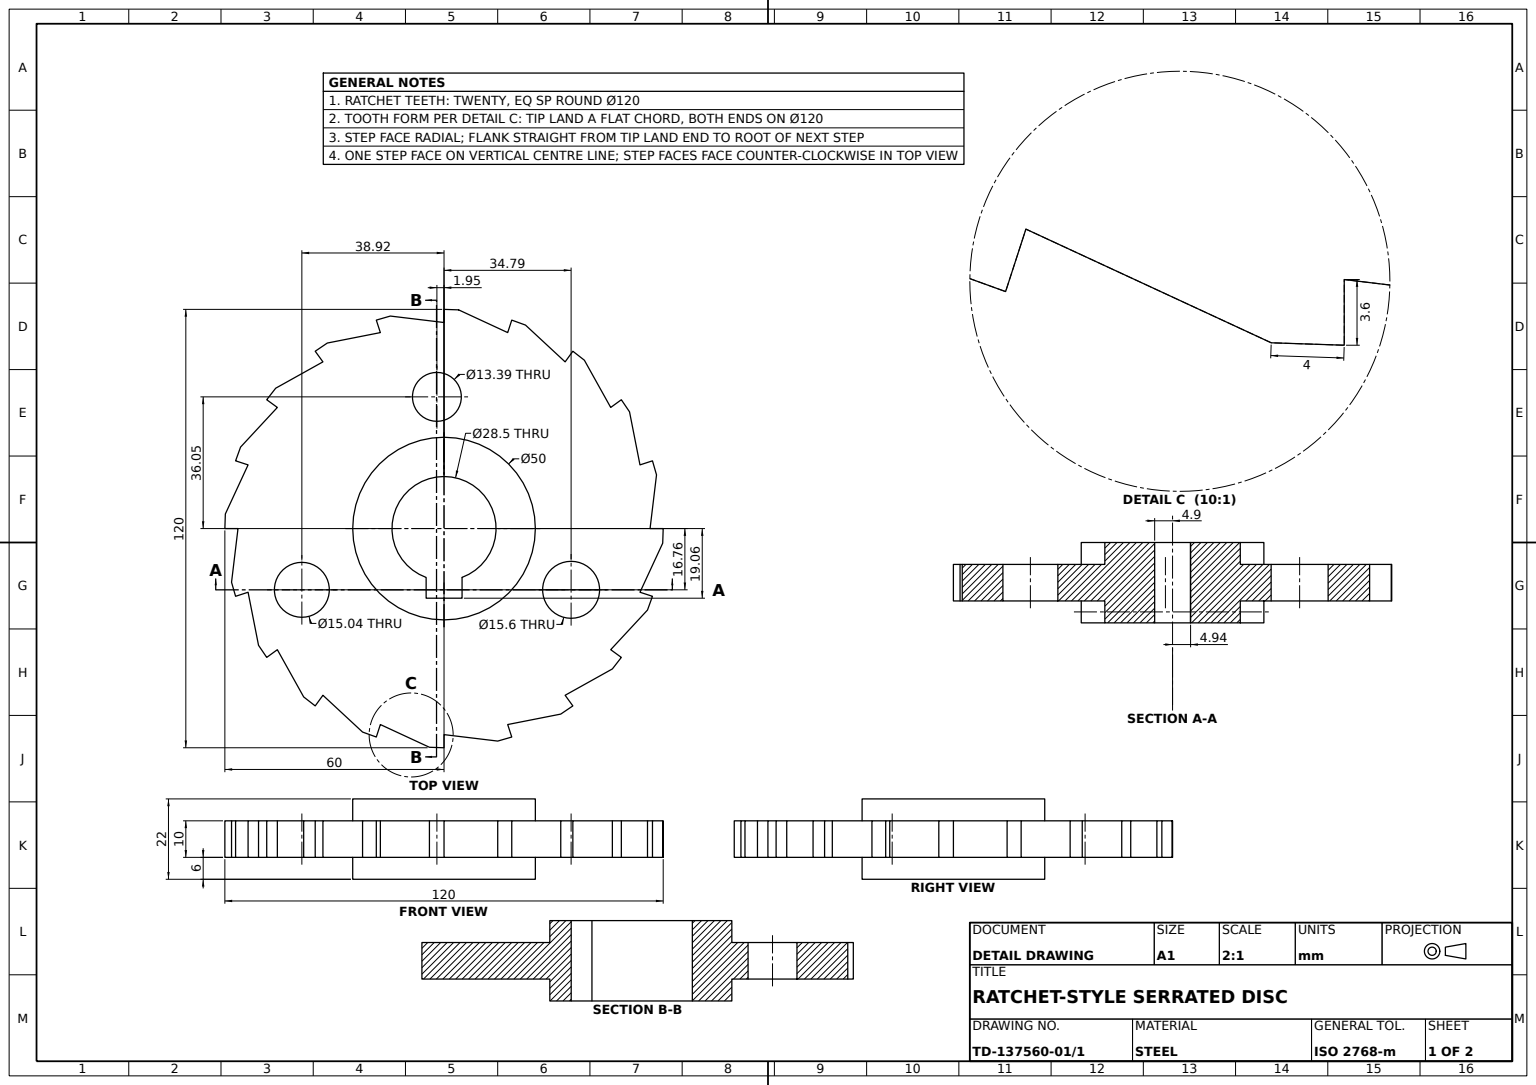
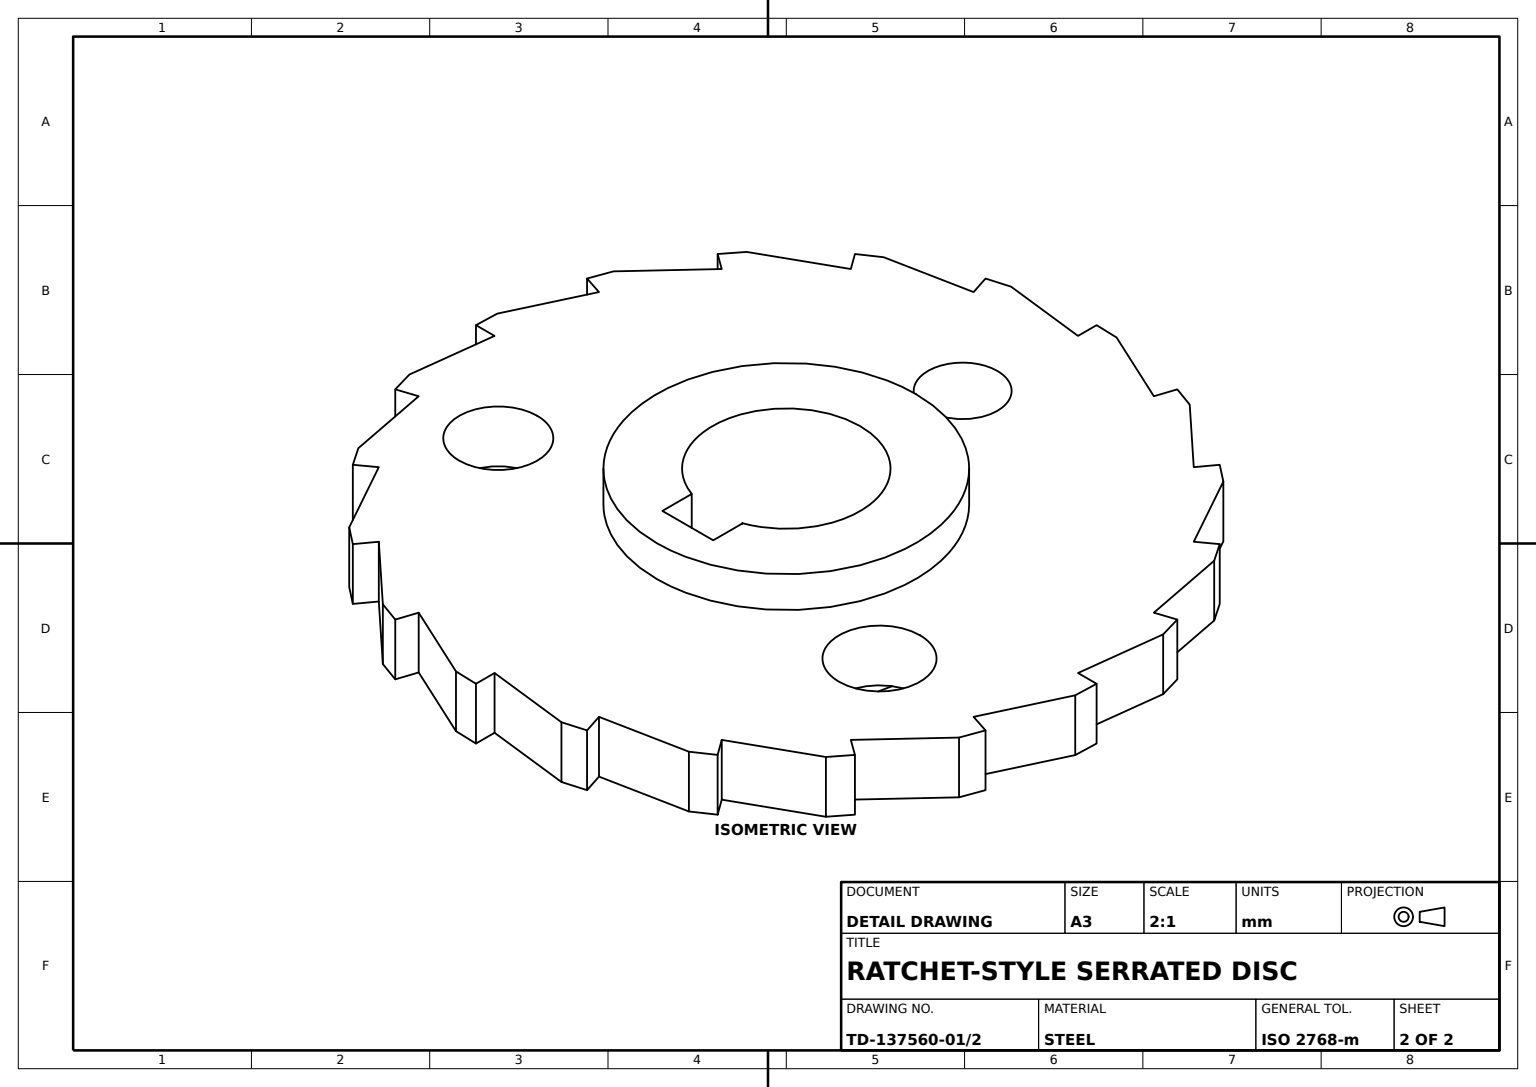
SolidWorks part; units mm, degrees
material "Plain Carbon Steel"
ref_plane "Front Plane" through (0, 0, 0) normal (0, 0, 1) x (1, 0, 0)
ref_plane "Top Plane" through (0, 0, 0) normal (0, 1, 0) x (1, 0, 0)
ref_plane "Right Plane" through (0, 0, 0) normal (1, 0, 0) x (0, 0, -1)
sketch "Ratchet Tooth Profile Sketch" plane through (0, 0, 0) normal (0, 1, 0) x (1, 0, 0)
  line L0 (0, -56) -> (0, -60)
  line L1 (0, -60) -> (3.9978, -59.8667)
  line L2 (3.9978, -59.8667) -> (17.4297, -53.6432)
  line L3 (23.8372, -54.2766) -> (23.9015, -55.0338)
  line L4 (-14.6977, -58.172) -> (0, -56.4038)
  line L5 (-18.541, -57.0634) -> (-14.6977, -58.172)
  line L6 (-17.305, -53.2592) -> (-18.541, -57.0634)
  line L7 (-31.9544, -50.783) -> (-17.4297, -53.6432)
  line L8 (-35.2671, -48.541) -> (-31.9544, -50.783)
  line L9 (-32.916, -45.305) -> (-35.2671, -48.541)
  line L10 (-46.0833, -38.423) -> (-33.1533, -45.6316)
  line L11 (-48.541, -35.2671) -> (-46.0833, -38.423)
  line L12 (-45.305, -32.916) -> (-48.541, -35.2671)
  line L13 (-55.7012, -22.302) -> (-45.6316, -33.1533)
  line L14 (-57.0634, -18.541) -> (-55.7012, -22.302)
  line L15 (-53.2592, -17.305) -> (-57.0634, -18.541)
  line L16 (-59.8667, -3.9978) -> (-53.6432, -17.4297)
  line L17 (-60, 0) -> (-59.8667, -3.9978)
  line L18 (-56, 0) -> (-60, 0)
  line L19 (-58.172, 14.6977) -> (-56.4038, 0)
  line L20 (-57.0634, 18.541) -> (-58.172, 14.6977)
  line L21 (-53.2592, 17.305) -> (-57.0634, 18.541)
  line L22 (-50.783, 31.9544) -> (-53.6432, 17.4297)
  line L23 (-48.541, 35.2671) -> (-50.783, 31.9544)
  line L24 (-45.305, 32.916) -> (-48.541, 35.2671)
  line L25 (-38.423, 46.0833) -> (-45.6316, 33.1533)
  line L26 (-35.2671, 48.541) -> (-38.423, 46.0833)
  line L27 (-32.916, 45.305) -> (-35.2671, 48.541)
  line L28 (-22.302, 55.7012) -> (-33.1533, 45.6316)
  line L29 (-18.541, 57.0634) -> (-22.302, 55.7012)
  line L30 (-17.305, 53.2592) -> (-18.541, 57.0634)
  line L31 (-3.9978, 59.8667) -> (-17.4297, 53.6432)
  line L32 (0, 60) -> (-3.9978, 59.8667)
  line L33 (0, 56) -> (0, 60)
  line L34 (14.6977, 58.172) -> (0, 56.4038)
  line L35 (18.541, 57.0634) -> (14.6977, 58.172)
  line L36 (17.305, 53.2592) -> (18.541, 57.0634)
  line L37 (31.9544, 50.783) -> (17.4297, 53.6432)
  line L38 (35.2671, 48.541) -> (31.9544, 50.783)
  line L39 (32.916, 45.305) -> (35.2671, 48.541)
  line L40 (46.0833, 38.423) -> (33.1533, 45.6316)
  line L41 (48.541, 35.2671) -> (46.0833, 38.423)
  line L42 (45.305, 32.916) -> (48.541, 35.2671)
  line L43 (55.7012, 22.302) -> (45.6316, 33.1533)
  line L44 (57.0634, 18.541) -> (55.7012, 22.302)
  line L45 (53.2592, 17.305) -> (57.0634, 18.541)
  line L46 (59.8667, 3.9978) -> (53.6432, 17.4297)
  line L47 (60, 0) -> (59.8667, 3.9978)
  line L48 (56, 0) -> (60, 0)
  line L49 (58.172, -14.6977) -> (56.4038, 0)
  line L50 (57.0634, -18.541) -> (58.172, -14.6977)
  line L51 (53.2592, -17.305) -> (57.0634, -18.541)
  line L52 (50.783, -31.9544) -> (53.6432, -17.4297)
  line L53 (48.541, -35.2671) -> (50.783, -31.9544)
  line L54 (45.305, -32.916) -> (48.541, -35.2671)
  line L55 (38.423, -46.0833) -> (45.6316, -33.1533)
  line L56 (35.2671, -48.541) -> (38.423, -46.0833)
  line L57 (32.916, -45.305) -> (35.2671, -48.541)
  line L58 (22.302, -55.7012) -> (33.1533, -45.6316)
  line L59 (18.541, -57.0634) -> (22.302, -55.7012)
  line L60 (17.305, -53.2592) -> (18.541, -57.0634)
  arc A0 (0, -60) -> (3.9978, -59.8667) centre (0, 0) ccw
  point P87 (0, 0)
  dimension "D1" = 120
  dimension "D2" = 3.9978
  dimension "D3" = 70
  dimension "D5" = 17.305
  dimension "D6" = 17.4297
  dimension "D7" = 23.8372
  dimension "D4" = 20
extrude "Ratchet Wheel Body 20T" add sketch "Ratchet Tooth Profile Sketch" along normal blind 10
sketch "Hub Sketch" plane through (0, 10, 0) normal (0, 1, 0) x (1, 0, 0)
  circle A0 centre (0, 0) radius 25
  dimension "D1" = 50
extrude "Hub Boss Ø50" add sketch "Hub Sketch" along normal blind 6 and the other way blind 16
sketch "Keyed Bore Sketch" plane through (0, 16, 0) normal (0, 1, 0) x (1, 0, 0)
  line L1 (4.8986, 13.3816) -> (4.9371, 13.3816)
  line L2 (-4.8986, 13.3816) -> (-4.8986, 19.0594)
  line L3 (-4.8986, 19.0594) -> (4.9371, 19.0594)
  line L4 (4.9371, 13.3816) -> (4.9371, 19.0594)
  arc A0 (-4.8986, 13.3816) -> (4.8986, 13.3816) centre (0, 0) ccw
  circle A1 centre (0, 0) radius 25 construction
  dimension "D1" = 28.5
  dimension "D2" = 4.8986
  dimension "D3" = 4.9371
  dimension "D4" = 19.0594
extrude "Keyed Shaft Bore" cut sketch "Keyed Bore Sketch" against normal blind 57
sketch "Through Holes Sketch" plane through (0, 0, 0) normal (0, 1, 0) x (1, 0, 0)
  circle A0 centre (-38.9224, 16.7631) radius 7.5219
  circle A1 centre (34.7891, 16.7631) radius 7.8007
  circle A2 centre (-1.9519, -36.052) radius 6.6948
  dimension "D1" = 15.0439
  dimension "D2" = 15.6014
  dimension "D3" = 13.3897
  dimension "D4" = 38.9224
  dimension "D5" = 16.7631
  dimension "D6" = 34.7891
  dimension "D7" = 1.9519
  dimension "D8" = 36.052
extrude "Through Holes 3x" cut sketch "Through Holes Sketch" against normal blind 57 and the other way blind 57
